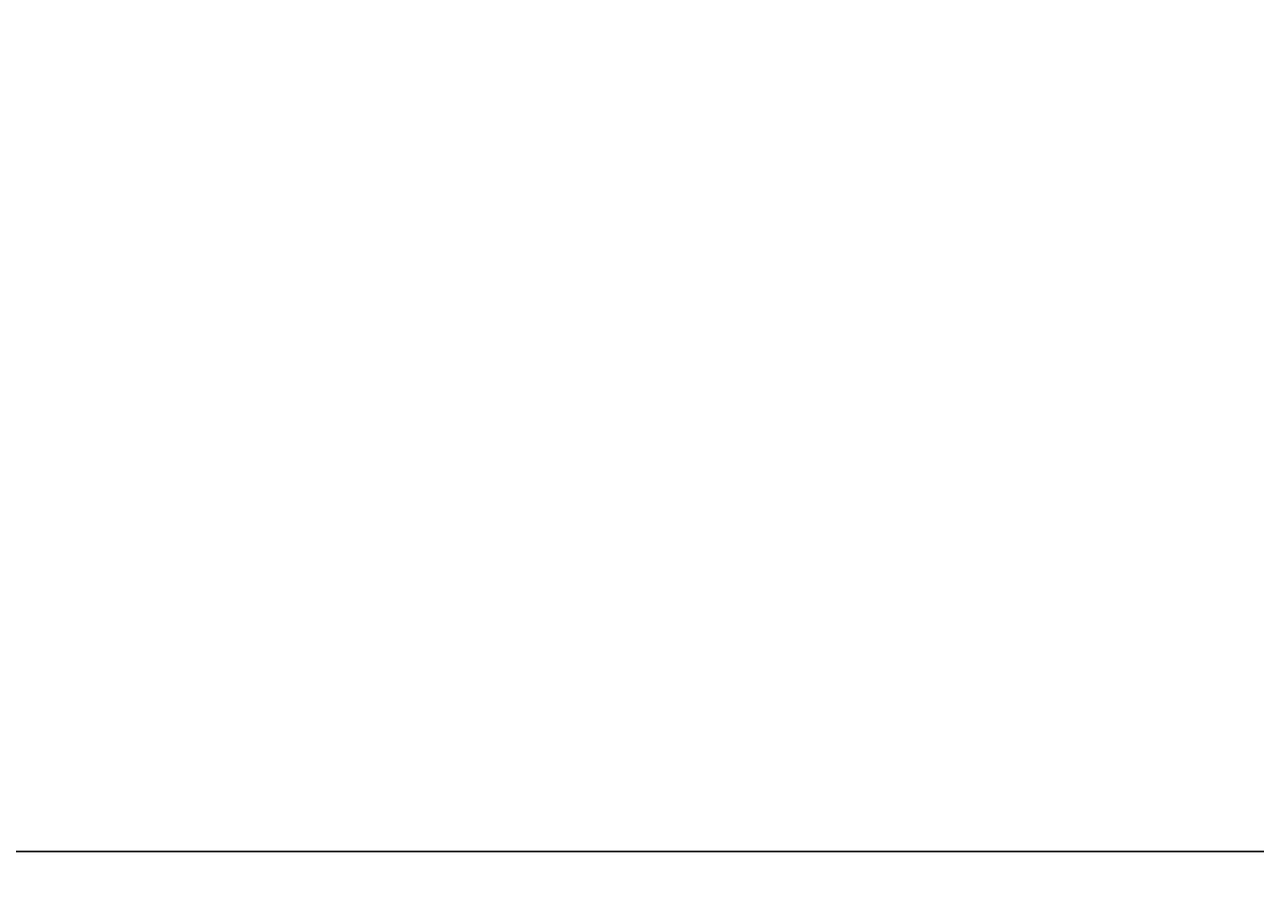
# Model space of a CAD drawing. Units: inches. Extents: x 35362 to 73946, y 43607 to 67532.
# Tile 110 of 134: x 50905 to 50977, y 48917 to 48969. Entities that reach past the tile are written whole.
import ezdxf

# ---------------------------------------------------------------- set-up
doc = ezdxf.new("R2010")
doc.units = ezdxf.units.IN
doc.header["$MEASUREMENT"] = 0
doc.layers.add('A-ANNO-DIMS', color=2, linetype='Continuous', lineweight=18)
doc.styles.get("Standard").update_dxf_attribs({"font": 'arial.ttf'})
doc.dimstyles.get("Standard").update_dxf_attribs({"dimtxt": 0.18, "dimasz": 0.18, "dimexe": 0.18, "dimexo": 0.0625, "dimgap": 0.09, "dimtad": 0, "dimtih": 1, "dimtoh": 1, "dimdec": 4, "dimzin": 0, "dimdsep": 46, "dimtxsty": 'Standard', "dimcen": 0.09, "dimadec": 0, "dimazin": 0, "dimtfac": 1, "dimtdec": 4, "dimtofl": 0, "dimtmove": 0, "dimatfit": 3, "dimfxl": 1, "dimtolj": 1, "dimtzin": 0, "dimarcsym": 0})

# ---------------------------------------------------------------- blocks, each defined once
blk = doc.blocks.new('*D11')
at = {"layer": 'A-ANNO-DIMS', "color": 0, "lineweight": -2, "transparency": 16777216}
for p, q in [((47978.665, 56028.774), (47978.665, 43606.679)), ((53109.76, 56028.774), (53109.76, 43606.679)), ((47978.845, 43606.859), (50543.871, 43606.859)), ((53109.58, 43606.859), (50544.554, 43606.859))]:
    blk.add_line(p, q, dxfattribs=at)
at = {"layer": 'A-ANNO-DIMS', "color": 0, "transparency": 16777216}
for points in [[(47978.845, 43606.889), (47978.845, 43606.829), (47978.665, 43606.859)], [(53109.58, 43606.889), (53109.58, 43606.829), (53109.76, 43606.859)]]:
    blk.add_solid(points, dxfattribs=at)
at = {"layer": 'Defpoints', "color": 0, "transparency": 16777216}
for p in [(47978.665, 56028.836), (53109.76, 56028.836), (53109.76, 43606.859)]:
    blk.add_point(p, dxfattribs=at)
at = {"layer": 'A-ANNO-DIMS', "color": 0, "transparency": 16777216, "insert": (50544.212, 43606.859), "char_height": 0.18, "attachment_point": 5}
blk.add_mtext('\\A1;5131', dxfattribs=at)
blk = doc.blocks.new('*D13')
at = {"layer": 'A-ANNO-DIMS', "color": 0, "lineweight": -2, "transparency": 16777216}
for p, q in [((48373.492, 51694.025), (48373.492, 43606.679)), ((51029.043, 51694.025), (51029.043, 43606.679)), ((48373.672, 43606.859), (49700.802, 43606.859)), ((51028.863, 43606.859), (49701.733, 43606.859))]:
    blk.add_line(p, q, dxfattribs=at)
at = {"layer": 'A-ANNO-DIMS', "color": 0, "transparency": 16777216}
for points in [[(48373.672, 43606.889), (48373.672, 43606.829), (48373.492, 43606.859)], [(51028.863, 43606.889), (51028.863, 43606.829), (51029.043, 43606.859)]]:
    blk.add_solid(points, dxfattribs=at)
at = {"layer": 'Defpoints', "color": 0, "transparency": 16777216}
for p in [(48373.492, 51694.087), (51029.043, 51694.087), (51029.043, 43606.859)]:
    blk.add_point(p, dxfattribs=at)
at = {"layer": 'A-ANNO-DIMS', "color": 0, "transparency": 16777216, "insert": (49701.267, 43606.859), "char_height": 0.18, "attachment_point": 5}
blk.add_mtext('\\A1;2655.6', dxfattribs=at)
blk = doc.blocks.new('*D17')
at = {"layer": 'A-ANNO-DIMS', "color": 0, "lineweight": -2, "transparency": 16777216}
for p, q in [((49923.307, 61293.224), (49923.307, 43606.679)), ((51913.931, 61293.224), (51913.931, 43606.679)), ((49923.487, 43606.859), (50918.164, 43606.859)), ((51913.751, 43606.859), (50919.074, 43606.859))]:
    blk.add_line(p, q, dxfattribs=at)
at = {"layer": 'A-ANNO-DIMS', "color": 0, "transparency": 16777216}
for points in [[(49923.487, 43606.889), (49923.487, 43606.829), (49923.307, 43606.859)], [(51913.751, 43606.889), (51913.751, 43606.829), (51913.931, 43606.859)]]:
    blk.add_solid(points, dxfattribs=at)
at = {"layer": 'Defpoints', "color": 0, "transparency": 16777216}
for p in [(49923.307, 61293.286), (51913.931, 61293.286), (51913.931, 43606.859)]:
    blk.add_point(p, dxfattribs=at)
at = {"layer": 'A-ANNO-DIMS', "color": 0, "transparency": 16777216, "insert": (50918.619, 43606.859), "char_height": 0.18, "attachment_point": 5}
blk.add_mtext('\\A1;1990.6', dxfattribs=at)
blk = doc.blocks.new('*D67')
at = {"layer": 'A-ANNO-DIMS', "color": 0, "lineweight": -2, "transparency": 16777216}
for p, q in [((56873.539, 53351.529), (35361.769, 53351.529)), ((35361.949, 53351.349), (35361.949, 49400.893)), ((35361.949, 45450.074), (35361.949, 49400.53)), ((53793.575, 45449.894), (35361.769, 45449.894))]:
    blk.add_line(p, q, dxfattribs=at)
at = {"layer": 'A-ANNO-DIMS', "color": 0, "transparency": 16777216}
for points in [[(35361.919, 53351.349), (35361.979, 53351.349), (35361.949, 53351.529)], [(35361.919, 45450.074), (35361.979, 45450.074), (35361.949, 45449.894)]]:
    blk.add_solid(points, dxfattribs=at)
at = {"layer": 'Defpoints', "color": 0, "transparency": 16777216}
for p in [(35361.949, 53351.529), (56873.602, 53351.529), (53793.638, 45449.894)]:
    blk.add_point(p, dxfattribs=at)
at = {"layer": 'A-ANNO-DIMS', "color": 0, "transparency": 16777216, "insert": (35361.949, 49400.712), "char_height": 0.18, "attachment_point": 5}
blk.add_mtext('\\A1;7901.6', dxfattribs=at)
blk = doc.blocks.new('*D86')
at = {"layer": 'A-ANNO-DIMS', "color": 0, "lineweight": -2, "transparency": 16777216}
for p, q in [((51285.532, 49320.079), (35361.769, 49320.079)), ((35361.949, 49319.899), (35361.949, 49120.261)), ((35361.949, 48920.259), (35361.949, 49119.897)), ((51285.532, 48920.079), (35361.769, 48920.079))]:
    blk.add_line(p, q, dxfattribs=at)
at = {"layer": 'A-ANNO-DIMS', "color": 0, "transparency": 16777216}
for points in [[(35361.919, 49319.899), (35361.979, 49319.899), (35361.949, 49320.079)], [(35361.919, 48920.259), (35361.979, 48920.259), (35361.949, 48920.079)]]:
    blk.add_solid(points, dxfattribs=at)
at = {"layer": 'Defpoints', "color": 0, "transparency": 16777216}
for p in [(35361.949, 49320.079), (51285.595, 49320.079), (51285.595, 48920.079)]:
    blk.add_point(p, dxfattribs=at)
at = {"layer": 'A-ANNO-DIMS', "color": 0, "transparency": 16777216, "insert": (35361.949, 49120.079), "char_height": 0.18, "attachment_point": 5}
blk.add_mtext('\\A1;400.0', dxfattribs=at)
blk = doc.blocks.new('*D107')
at = {"layer": 'A-ANNO-DIMS', "color": 0, "lineweight": -2, "transparency": 16777216}
for p, q in [((50139.563, 59850.014), (50139.563, 43606.679)), ((51320.813, 59850.014), (51320.813, 43606.679)), ((50139.743, 43606.859), (50729.733, 43606.859)), ((51320.633, 43606.859), (50730.643, 43606.859))]:
    blk.add_line(p, q, dxfattribs=at)
at = {"layer": 'A-ANNO-DIMS', "color": 0, "transparency": 16777216}
for points in [[(50139.743, 43606.889), (50139.743, 43606.829), (50139.563, 43606.859)], [(51320.633, 43606.889), (51320.633, 43606.829), (51320.813, 43606.859)]]:
    blk.add_solid(points, dxfattribs=at)
at = {"layer": 'Defpoints', "color": 0, "transparency": 16777216}
for p in [(50139.563, 59850.077), (51320.813, 59850.077), (51320.813, 43606.859)]:
    blk.add_point(p, dxfattribs=at)
at = {"layer": 'A-ANNO-DIMS', "color": 0, "transparency": 16777216, "insert": (50730.188, 43606.859), "char_height": 0.18, "attachment_point": 5}
blk.add_mtext('\\A1;1181.3', dxfattribs=at)

msp = doc.modelspace()

# ---------------------------------------------------------------- dimensions: what is measured, and where the dimension line sits
at = {"layer": 'A-ANNO-DIMS'}
for base, p1, p2, override, picture, middle in [((51913.931, 43606.859), (49923.307, 61293.286), (51913.931, 61293.286), {"dimdec": 1, "dimlfac": 1, "dimrnd": 0, "dimzin": 0, "dimdsep": 46, "dimlunit": 2}, '*D17', (50918.619, 43606.859)), ((51320.8133, 43606.859), (50139.5627, 59850.0769), (51320.8133, 59850.0769), {"dimdec": 1, "dimlfac": 1, "dimrnd": 0, "dimzin": 0, "dimdsep": 46, "dimlunit": 2}, '*D107', (50730.188, 43606.859)), ((53109.76, 43606.859), (47978.665, 56028.836), (53109.76, 56028.836), {"dimdec": 0, "dimlfac": 1, "dimrnd": 0, "dimzin": 0, "dimdsep": 46, "dimlunit": 2}, '*D11', (50544.212, 43606.859)), ((51029.043, 43606.859), (48373.492, 51694.087), (51029.043, 51694.087), {"dimdec": 1, "dimlfac": 1, "dimrnd": 0, "dimzin": 0, "dimdsep": 46, "dimlunit": 2}, '*D13', (49701.267, 43606.859))]:
    dim = msp.add_linear_dim(base=base, p1=p1, p2=p2, dimstyle='Standard', override=override, dxfattribs=at)
    dim.commit()
    dim.dimension.update_dxf_attribs({"geometry": picture, "text_midpoint": middle})
for base, p1, p2, picture, middle in [((35361.949, 53351.529), (53793.638, 45449.894), (56873.602, 53351.529), '*D67', (35361.949, 49400.712)), ((35361.949, 49320.079), (51285.595, 48920.079), (51285.595, 49320.079), '*D86', (35361.949, 49120.079))]:
    dim = msp.add_linear_dim(base=base, p1=p1, p2=p2, angle=90, dimstyle='Standard', override={"dimdec": 1, "dimlfac": 1, "dimrnd": 0, "dimzin": 0, "dimdsep": 46, "dimlunit": 2}, dxfattribs=at)
    dim.commit()
    dim.dimension.update_dxf_attribs({"geometry": picture, "text_midpoint": middle})

doc.saveas('drawing.dxf')
